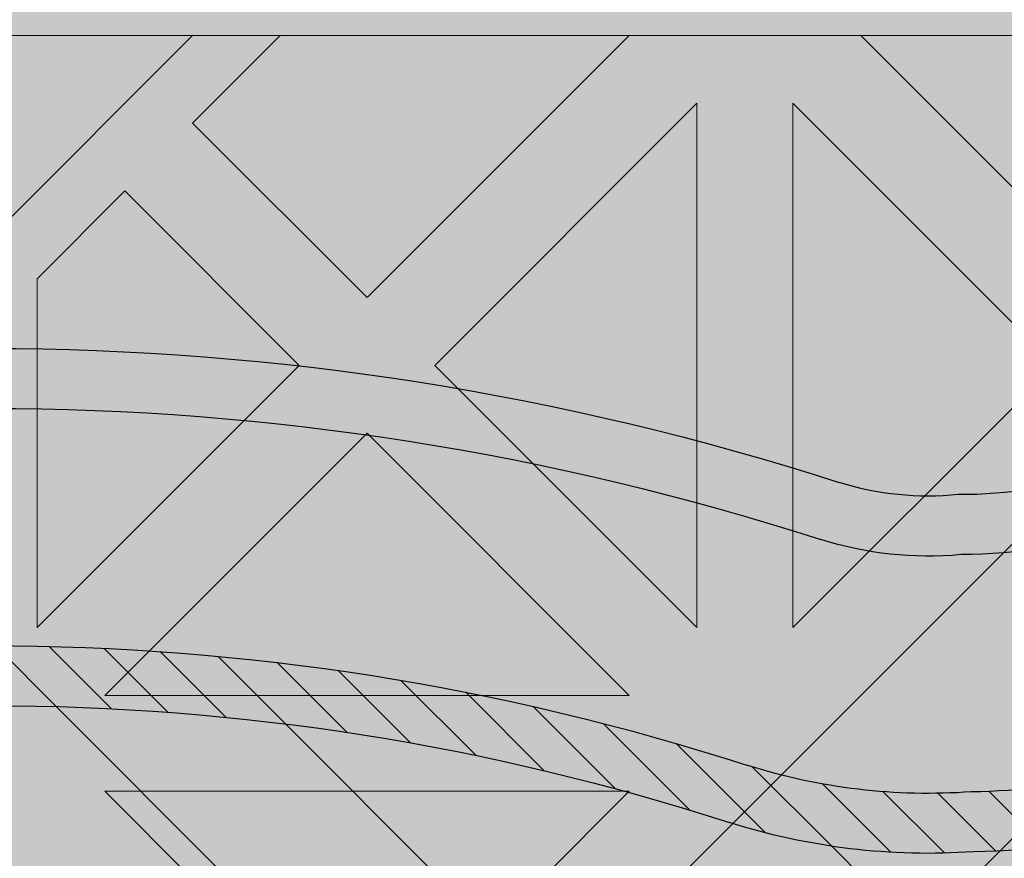
# Model space of a CAD drawing. Units: inches. Extents: x 844 to 2234, y 346 to 1084.
# Tile 81 of 93: x 2003.94 to 2006.557, y 708.742 to 710.971. Entities that reach past the tile are written whole.
import ezdxf

# ---------------------------------------------------------------- set-up
doc = ezdxf.new("R2010")
doc.units = ezdxf.units.IN
doc.header["$MEASUREMENT"] = 0
for name, color, linetype, lineweight in [('A-ANNO-DIMS', 2, 'Continuous', 18), ('furniture', 8, 'Continuous', 18), ('RA-AP-01$0$INT', 35, 'Continuous', 5)]:
    doc.layers.add(name, color=color, linetype=linetype, lineweight=lineweight)
doc.layers.add('RA-AP-01$0$FURN', color=3, linetype='Continuous')
doc.layers.add('RA-AP-01$0$WOOD', color=64, linetype='Continuous')
doc.styles.get("Standard").update_dxf_attribs({"font": 'arial.ttf'})
doc.dimstyles.get("Standard").update_dxf_attribs({"dimtxt": 6, "dimasz": 3, "dimexe": 0.18, "dimexo": 0.0625, "dimgap": 0.09, "dimtad": 0, "dimtih": 1, "dimtoh": 1, "dimdec": 1, "dimzin": 0, "dimdsep": 46, "dimlunit": 3, "dimtxsty": 'Standard', "dimblk": 'ARCHTICK', "dimcen": 0.09, "dimadec": 0, "dimazin": 0, "dimtfac": 1, "dimtdec": 1, "dimtofl": 0, "dimtmove": 0, "dimatfit": 3, "dimfxl": 1, "dimtolj": 1, "dimtzin": 0, "dimarcsym": 0})

# ---------------------------------------------------------------- blocks, each defined once
blk = doc.blocks.new('A$C18D01794')
at = {"layer": 'RA-AP-01$0$INT'}
blk.add_hatch(color=256, dxfattribs=at).paths.add_polyline_path([(4.505206456958071, -7.906712009588039), (5.305206456958072, -7.906712009588039), (5.305206456958072, -7.106712009588038), (5.255206456951893, -7.106712009588036), (5.25520645694868, -7.856712009570104), (4.555206456959269, -7.856712009588616), (4.555206456956052, -7.106712009588038), (4.505206456958073, -7.106712009588038)])
h = blk.add_hatch(color=256, dxfattribs=at)
h.paths.add_polyline_path([(4.585917135068448, -7.856712009587804), (4.614201406330596, -7.856712009587056), (4.668846067270487, -7.802067348644738), (4.723490728212344, -7.856712009584164), (4.771774999457151, -7.856712009582887), (4.826419660396886, -7.80206734864072), (4.862780050090322, -7.838427738332541), (4.844495778842715, -7.856712009580965), (4.862780050090411, -7.856712009580482), (4.905206456960182, -7.814285602707865), (4.947632863832445, -7.856712009578238), (4.965917135079675, -7.856712009577755), (4.947632863831759, -7.838427738330656), (4.983993253523576, -7.802067348637219), (5.038637914464627, -7.856712009575829), (5.08692218571208, -7.856712009574554), (5.141566846649976, -7.802067348634224), (5.196211507589851, -7.856712009571666), (5.224495778822615, -7.856712009570916), (4.905206456953975, -7.537422687702283)])
h.paths.add_polyline_path([(4.895206456956031, -7.575706958950402), (4.895206456958921, -7.684996280828174), (4.840561796018589, -7.630351619890275)], flags=16)
h.paths.add_polyline_path([(4.915206456955638, -7.575706958949956), (4.969851117895509, -7.630351619887399), (4.915206456957609, -7.684996280827732)], flags=16)
h.paths.add_polyline_path([(4.826419660395175, -7.644493755514321), (4.881064321335613, -7.699138416452331), (4.771774999456703, -7.69913841645522)], flags=16)
h.paths.add_polyline_path([(4.983993253519558, -7.644493755510815), (5.038637914460456, -7.699138416449285), (4.929348592581548, -7.69913841645126)], flags=16)
h.paths.add_polyline_path([(4.881064321336025, -7.719138416452334), (4.826419660397532, -7.773783077393256), (4.771774999457062, -7.719138416455217)], flags=16)
h.paths.add_polyline_path([(4.929348592582019, -7.71913841645126), (5.038637914460982, -7.719138416449284), (4.983993253522945, -7.773783077389749)], flags=16)
h.paths.add_polyline_path([(4.895206456960191, -7.733280552075633), (4.895206456962115, -7.806001331460164), (4.876922185715016, -7.824285602708492), (4.840561796021581, -7.787925213016675)], flags=16)
h.paths.add_polyline_path([(4.915206456958487, -7.733280552075187), (4.969851117899527, -7.787925213013798), (4.933490728206909, -7.824285602708034), (4.9152064569598, -7.806001331461736)], flags=16)
h.paths.add_polyline_path([(4.757632863832376, -7.733280552079264), (4.812277524772842, -7.787925213017304), (4.757632863834348, -7.842569873958233)], flags=16)
h.paths.add_polyline_path([(4.737632863832376, -7.73328055207979), (4.737632863834348, -7.842569873958701), (4.682988202893906, -7.787925213020692)], flags=16)
h.paths.add_polyline_path([(5.05278005008503, -7.733280552072701), (5.052780050087917, -7.842569873951664), (4.998135389146995, -7.787925213013169)], flags=16)
h.paths.add_polyline_path([(5.072780050085024, -7.733280552072333), (5.127424711025931, -7.787925213010806), (5.072780050087916, -7.842569873951244)], flags=16)
h.paths.add_polyline_path([(4.935917135072783, -7.506712009583784), (5.255206456948811, -7.826001331459767), (5.255206456948932, -7.797717060211899), (5.200561796010279, -7.743072399273238), (5.255206456949403, -7.688427738334128), (5.25520645694961, -7.640143467086677), (5.200561796009787, -7.585498806146837), (5.236922185702417, -7.549138416454212), (5.255206456949919, -7.56742268770172), (5.255206456949998, -7.549138416454178), (5.212780050078687, -7.506712009583814), (5.25520645695036, -7.464285602712145), (5.255206456950438, -7.446001331464763), (5.236922185702424, -7.464285602712779), (5.200561796009796, -7.427925213020149), (5.255206456950753, -7.373280552079203), (5.25520645695096, -7.324996280834394), (5.200561796010322, -7.270351619893748), (5.255206456951428, -7.215706958952649), (5.255206456951547, -7.187422687705071)])
h.paths.add_polyline_path([(5.042988202883395, -7.42792521302065), (5.097632863823085, -7.373280552080975), (5.097632863822622, -7.482569873959883)], flags=16)
h.paths.add_polyline_path([(5.028846067259663, -7.442067348644384), (5.083490728198774, -7.496712009583504), (4.974201406321001, -7.496712009583035)], flags=16)
h.paths.add_polyline_path([(5.117632863823087, -7.37328055208089), (5.172277524762331, -7.42792521302015), (5.11763286382262, -7.482569873959851)], flags=16)
h.paths.add_polyline_path([(5.08349072819877, -7.516712009582191), (5.028846067259652, -7.571356670521302), (4.974201406320998, -7.516712009582638)], flags=16)
h.paths.add_polyline_path([(5.131774999446817, -7.35913841645716), (5.186419660386065, -7.413783077396415), (5.241064321325782, -7.359138416456712)], flags=17)
h.paths.add_polyline_path([(5.131774999446228, -7.496712009583703), (5.186419660386065, -7.442067348643883), (5.222780050079488, -7.478427738337313), (5.204495778832781, -7.496712009584014)], flags=16)
h.paths.add_polyline_path([(5.097632863822613, -7.530854145205813), (5.097632863823061, -7.640143467084723), (5.042988202883383, -7.585498806145032)], flags=16)
h.paths.add_polyline_path([(5.131774999446899, -7.339138416457162), (5.241064321325809, -7.339138416456712), (5.186419660386591, -7.284493755517479)], flags=17)
h.paths.add_polyline_path([(5.131774999446226, -7.516712009581999), (5.204495778830767, -7.516712009581702), (5.22278005007868, -7.534996280829206), (5.186419660386049, -7.571356670521828)], flags=16)
h.paths.add_polyline_path([(5.11763286382262, -7.530854145205852), (5.17227752476232, -7.585498806145562), (5.117632863823064, -7.64014346708481)], flags=16)
h.paths.add_polyline_path([(5.186419660386069, -7.599640941770585), (5.241064321325754, -7.654285602710281), (5.131774999446791, -7.654285602709814)], flags=16)
h.paths.add_polyline_path([(5.131774999446872, -7.674285602709813), (5.24106432132578, -7.674285602710282), (5.186419660386554, -7.728930263649504)], flags=16)
h.paths.add_polyline_path([(5.255206456951811, -7.126001331467467), (5.255206456951895, -7.106712009588038), (4.555206456956052, -7.106712009588038), (4.555206456956136, -7.12600133146746), (4.905206456953973, -7.476001331465289)])
h.paths.add_polyline_path([(4.983993253513404, -7.368930263651977), (4.92934859257295, -7.314285602713969), (5.03863791445186, -7.314285602711063)], flags=16)
h.paths.add_polyline_path([(4.969851117889988, -7.383072399276016), (4.915206456952556, -7.437717060215906), (4.915206456949648, -7.328427738338133)], flags=16)
h.paths.add_polyline_path([(4.929348592572535, -7.294285602713971), (4.983993253511019, -7.239640941773039), (5.038637914451496, -7.294285602711065)], flags=16)
h.paths.add_polyline_path([(5.052780050074912, -7.280143467087016), (4.998135389134438, -7.225498806148989), (5.052780050072919, -7.170854145208052)], flags=16)
h.paths.add_polyline_path([(5.07278005007491, -7.280143467086489), (5.072780050072918, -7.170854145207579), (5.127424711013374, -7.225498806145578)], flags=16)
h.paths.add_polyline_path([(4.89520645695295, -7.437717060216355), (4.840561796013067, -7.383072399278919), (4.895206456950961, -7.328427738338582)], flags=16)
h.paths.add_polyline_path([(4.915206456948365, -7.280143467090674), (4.915206456946434, -7.207422687704125), (4.933490728192729, -7.18913841645701), (4.969851117886972, -7.225498806149623)], flags=16)
h.paths.add_polyline_path([(4.881064321327021, -7.314285602715054), (4.82641966038902, -7.368930263655506), (4.771774999448108, -7.314285602717047)], flags=16)
h.paths.add_polyline_path([(4.895206456950073, -7.280143467091125), (4.840561796009022, -7.225498806152518), (4.876922185700835, -7.18913841645908), (4.895206456948749, -7.207422687706589)], flags=16)
h.paths.add_polyline_path([(4.983993253510392, -7.211356670525576), (4.947632863816944, -7.174996280833758), (4.965917135064043, -7.156712009585847), (5.038637914448995, -7.156712009584522)], flags=16)
h.paths.add_polyline_path([(4.881064321326543, -7.294285602715056), (4.771774999447578, -7.294285602717046), (4.826419660385607, -7.239640941776569)], flags=16)
h.paths.add_polyline_path([(4.905206456946447, -7.19913841645844), (4.862780050074785, -7.156712009587725), (4.947632863816685, -7.156712009586302)], flags=16)
h.paths.add_polyline_path([(5.14156684663679, -7.211356670521528), (5.086922185696452, -7.156712009583639), (5.196211507574223, -7.156712009581651)], flags=16)
h.paths.add_polyline_path([(4.8264196603837, -7.211356670529104), (4.771774999442643, -7.156712009590501), (4.8444957788276, -7.156712009588568), (4.862780050075511, -7.17499628083566)], flags=16)
h.paths.add_polyline_path([(4.812277524760289, -7.225498806153156), (4.757632863822258, -7.28014346709363), (4.757632863819352, -7.170854145214669)], flags=16)
h.paths.add_polyline_path([(4.73763286382226, -7.280143467093997), (4.682988202881349, -7.22549880615554), (4.737632863819352, -7.170854145215086)], flags=16)
h.paths.add_polyline_path([(4.723490728195188, -7.156712009591787), (4.668846067257299, -7.211356670532127), (4.614201406317417, -7.156712009594693)], flags=16)
h.paths.add_polyline_path([(4.597632863829262, -7.506712009583814), (4.555206456957951, -7.54913841645418), (4.555206456958029, -7.56742268770172), (4.573490728205535, -7.549138416454212), (4.609851117898167, -7.585498806146839), (4.555206456958338, -7.640143467086675), (4.555206456958546, -7.688427738334125), (4.60985111789767, -7.743072399273238), (4.555206456959015, -7.797717060211899), (4.555206456959138, -7.826001331459767), (4.874495778835167, -7.506712009583786), (4.5552064569564, -7.187422687705062), (4.555206456956523, -7.215706958952644), (4.609851117897629, -7.270351619893746), (4.555206456956988, -7.324996280834396), (4.555206456957198, -7.373280552079195), (4.609851117898153, -7.427925213020147), (4.573490728205528, -7.464285602712779), (4.555206456957507, -7.446001331464756), (4.555206456957585, -7.464285602712143)])
h.paths.add_polyline_path([(4.712780050085332, -7.482569873959882), (4.712780050084863, -7.373280552080972), (4.767424711024555, -7.42792521302065)], flags=16)
h.paths.add_polyline_path([(4.726922185709173, -7.496712009583504), (4.781566846648288, -7.442067348644384), (4.836211507586949, -7.496712009583033)], flags=16)
h.paths.add_polyline_path([(4.692780050085327, -7.482569873959851), (4.638135389145619, -7.427925213020149), (4.692780050084865, -7.373280552080892)], flags=16)
h.paths.add_polyline_path([(4.726922185709182, -7.516712009582191), (4.836211507586949, -7.51671200958264), (4.7815668466483, -7.571356670521304)], flags=16)
h.paths.add_polyline_path([(4.678637914461726, -7.496712009583706), (4.605917135075169, -7.496712009584014), (4.587632863828464, -7.478427738337311), (4.623993253521887, -7.442067348643881)], flags=16)
h.paths.add_polyline_path([(4.712780050085336, -7.530854145205816), (4.767424711024568, -7.585498806145034), (4.71278005008489, -7.640143467084724)], flags=16)
h.paths.add_polyline_path([(4.678637914461726, -7.516712009582001), (4.623993253521899, -7.571356670521829), (4.587632863829271, -7.534996280829206), (4.605917135077185, -7.5167120095817)], flags=16)
h.paths.add_polyline_path([(4.692780050085336, -7.530854145205848), (4.692780050084889, -7.64014346708481), (4.638135389145632, -7.585498806145562)], flags=16)
h.paths.add_polyline_path([(4.623993253521885, -7.413783077396415), (4.678637914461131, -7.359138416457161), (4.56934859258217, -7.359138416456712)], flags=17)
h.paths.add_polyline_path([(4.623993253521901, -7.599640941770568), (4.678637914461158, -7.654285602709814), (4.569348592582195, -7.654285602710281)], flags=16)
h.paths.add_polyline_path([(4.678637914461051, -7.339138416457162), (4.623993253521361, -7.284493755517479), (4.569348592582143, -7.339138416456712)], flags=17)
h.paths.add_polyline_path([(4.678637914461076, -7.674285602709813), (4.623993253521399, -7.728930263649504), (4.569348592582167, -7.674285602710281)], flags=16)
h = blk.add_hatch(color=256, dxfattribs=at)
h.paths.add_polyline_path([(4.905206456954232, -7.537422687702028), (4.874495778835232, -7.506712009583718), (4.555206456959138, -7.826001331459766), (4.555206456959269, -7.856712009588616), (4.585917135068449, -7.856712009587804)])
h.paths.add_polyline_path([(4.935917135072152, -7.506712009583152), (4.905206456953497, -7.537422687701806), (5.224495778822614, -7.856712009570917), (5.255206456948681, -7.856712009570104), (5.255206456948813, -7.826001331459768)])
h.paths.add_polyline_path([(5.255206456951549, -7.18742268770507), (5.255206456951813, -7.126001331467461), (4.905206456953563, -7.476001331465701), (4.935917135072559, -7.506712009584006)])
h.paths.add_polyline_path([(4.874495778835167, -7.506712009583785), (4.905206456953818, -7.476001331465132), (4.555206456956135, -7.126001331467458), (4.555206456956399, -7.187422687705064)])
h = blk.add_hatch(color=256, dxfattribs=at)
h.paths.add_polyline_path([(4.969851117891331, -7.630351619889621), (4.915206456952669, -7.575706958950966), (4.915206456952222, -7.684996280828739)])
h.paths.add_polyline_path([(4.895206456953064, -7.575706958950968), (4.840561796014413, -7.630351619889628), (4.895206456953533, -7.684996280828741)])
h.paths.add_polyline_path([(4.826419660390684, -7.644493755513362), (4.771774999451003, -7.699138416453052), (4.881064321329913, -7.699138416452587)])
h.paths.add_polyline_path([(4.881064321329884, -7.719138416452585), (4.771774999450921, -7.719138416453052), (4.82641966039018, -7.773783077392298)])
h.paths.add_polyline_path([(4.895206456953734, -7.733280552076196), (4.840561796013912, -7.787925213016031), (4.876922185707337, -7.824285602709455), (4.895206456954043, -7.806001331462747)])
h.paths.add_polyline_path([(4.862780050082808, -7.838427738332388), (4.826419660390178, -7.802067348639763), (4.771774999450351, -7.856712009579595), (4.844495778835303, -7.856712009579895)])
h.paths.add_polyline_path([(4.812277524766446, -7.787925213016036), (4.757632863827191, -7.733280552076788), (4.757632863826741, -7.842569873955747)])
h.paths.add_polyline_path([(4.737632863827191, -7.733280552076863), (4.682988202887508, -7.787925213016558), (4.737632863826743, -7.842569873955778)])
h.paths.add_polyline_path([(4.668846067263777, -7.802067348640287), (4.614201406325123, -7.856712009578949), (4.723490728202894, -7.856712009579402)])
h.paths.add_polyline_path([(4.905206456953846, -7.814285602708654), (4.862780050082654, -7.856712009579847), (4.947632863824561, -7.85671200958032)])
h.paths.add_polyline_path([(4.915206456952028, -7.733280552076195), (4.91520645695173, -7.806001331460731), (4.933490728199234, -7.824285602708648), (4.96985111789186, -7.787925213016022)])
h.paths.add_polyline_path([(5.038637914454841, -7.719138416453029), (4.929348592575874, -7.71913841645258), (4.983993253515593, -7.773783077392289)])
h.paths.add_polyline_path([(4.983993253515065, -7.644493755513352), (4.929348592575849, -7.699138416452582), (5.038637914454755, -7.699138416453031)])
h.paths.add_polyline_path([(5.052780050079843, -7.73328055207676), (4.998135389140595, -7.787925213016018), (5.052780050080309, -7.842569873955721)])
h.paths.add_polyline_path([(4.983993253516868, -7.802067348639752), (4.947632863824241, -7.838427738332383), (4.965917135071747, -7.856712009579888), (5.038637914456701, -7.856712009579572)])
h.paths.add_polyline_path([(5.127424711019533, -7.787925213016519), (5.072780050079843, -7.733280552076838), (5.07278005008031, -7.842569873955751)])
h.paths.add_polyline_path([(5.141566846643269, -7.802067348640248), (5.086922185704154, -7.85671200957937), (5.196211507581929, -7.856712009578901)])
for p, q in [((4.874495778835167, -7.506712009583786), (4.555206456959136, -7.826001331459769)), ((4.905206456953975, -7.537422687702283), (4.585917135071132, -7.856712009585121)), ((4.826419660395171, -7.644493755514321), (4.771774999456703, -7.69913841645522)), ((4.881064321335613, -7.699138416452333), (4.826419660395173, -7.64449375551432)), ((4.771774999456703, -7.69913841645522), (4.881064321335613, -7.699138416452333)), ((4.771774999457064, -7.719138416455219), (4.881064321336027, -7.719138416452333)), ((4.771774999457064, -7.719138416455219), (4.826419660397532, -7.773783077393256)), ((4.881064321336027, -7.719138416452333), (4.826419660397532, -7.773783077393256)), ((4.682988202893908, -7.78792521302069), (4.737632863832376, -7.733280552079792)), ((4.737632863832376, -7.733280552079792), (4.737632863834348, -7.842569873958701)), ((4.757632863832376, -7.733280552079266), (4.812277524772842, -7.787925213017302)), ((4.757632863832376, -7.733280552079266), (4.757632863834348, -7.842569873958229)), ((4.895206456960191, -7.73328055207563), (4.840561796021581, -7.787925213016675)), ((4.895206456962113, -7.806001331460581), (4.895206456960191, -7.73328055207563)), ((4.737632863834348, -7.842569873958701), (4.682988202893906, -7.787925213020692)), ((4.757632863834348, -7.842569873958229), (4.812277524772842, -7.787925213017302)), ((4.840561796021581, -7.787925213016674), (4.876922185715016, -7.824285602708492)), ((4.723490728210815, -7.856712009582635), (4.668846067270487, -7.802067348644737)), ((4.771774999458274, -7.856712009581762), (4.826419660396887, -7.80206734864072)), ((4.826419660396886, -7.80206734864072), (4.862780050090322, -7.838427738332541)), ((4.895206456959797, -7.806001331462484), (4.876922185715016, -7.824285602708492)), ((4.905206456960184, -7.814285602707865), (4.862780050090411, -7.856712009580478)), ((4.844495778843225, -7.856712009580453), (4.862780050090324, -7.838427738332541)), ((4.555206456959269, -7.856712009588616), (5.255206456948681, -7.856712009570104)), ((4.844495778843225, -7.856712009580451), (4.771774999458274, -7.856712009581762)), ((4.947632863832319, -7.856712009578112), (4.862780050090411, -7.856712009580478))]:
    blk.add_line(p, q, dxfattribs=at)
blk = doc.blocks.new('A$C32926AE1')
at = {"layer": 'RA-AP-01$0$WOOD'}
h = blk.add_hatch(color=256, dxfattribs=at)
h.dxf.hatch_style = 1
h.paths.add_polyline_path([(5.157430609644524, 4.573483066760929, -0.1009492694046607), (5.155401577623758, 4.593365984175333, -0.1842662638101597), (5.172249623284174, 4.638795604568598, 0.2056608120311276), (5.179560981299304, 4.661316324430096, 0.3614336704623542), (5.134352340494423, 4.706524965234944, 0.2056608120311297), (5.111831620632933, 4.699213607219793, -0.1842662638101113), (5.066402000239693, 4.682365561559342, -0.1055311479399994), (5.045656153913092, 4.68467289944697, 0.1567636581983829), (4.763886414745334, 4.684672899446966, -0.1055311479399895), (4.743140568418733, 4.68236556155934, -0.1842662638100833), (4.6977109480255, 4.69921360721979, 0.2056608120302612), (4.675190228164109, 4.706524965234949, 0.3614336704708441), (4.629981587358889, 4.66131632442871, 0.2056608120245944), (4.637292945374126, 4.638795604567974, -0.1842662638101024), (4.654140991034615, 4.59336598417475, -0.1009492694055169), (4.652111959013835, 4.573483066760181, 0.021410119221476), (4.629748025606143, 4.156712009541676, 0.0214101192214795), (4.652111959013809, 3.739940952323101, -0.1009492694059586), (4.654140991034615, 3.720058034908448, -0.1842662638100975), (4.637292945374126, 3.674628414515226, 0.2056608120245705), (4.629981587358889, 3.652107694654492, 0.3614336704708879), (4.675190228164113, 3.606899053848249, 0.2056608120302384), (4.697710948025501, 3.614210411863408, -0.1842662638100995), (4.743140568418738, 3.63105845752386, -0.1055311479402541), (4.763886414745388, 3.628751119636215, 0.1567636581983776), (5.045656153913137, 3.628751119636244, -0.1055311479397538), (5.066402000239692, 3.631058457523857, -0.1842662638101067), (5.111831620632931, 3.614210411863407, 0.2056608120310924), (5.134352340494417, 3.606899053848256, 0.3614336704624001), (5.179560981299307, 3.652107694653103, 0.2056608120311314), (5.172249623284175, 3.6746284145146, -0.1842662638101402), (5.155401577623758, 3.72005803490786, -0.1009492694051366), (5.15743060964455, 3.739940952322354, 0.0214101192215073), (5.179794543052287, 4.156712009541468, 0.0214101192215252)])
h.paths.add_polyline_path([(4.639748609479751, 4.156712009541513, 0.0213537860821624), (4.661970494867118, 3.741887061152232, -0.094075836301374), (4.664143710413708, 3.7196126951003, -0.1824818158568985), (4.644813765429836, 3.668037719127816, 0.2056608120245319), (4.639939526753007, 3.653023905887301, 0.3614336704710246), (4.676106439397173, 3.616856993242342, 0.2056608120302234), (4.691120252638095, 3.621731231919122, -0.1824818158602558), (4.742695228611606, 3.641061176902986, -0.1029891339458722), (4.766991894714349, 3.638256818950944, 0.156709409989566), (5.042550673941472, 3.638256818950105, -0.102989133958497), (5.066847340047078, 3.641061176902949, -0.1824818158594995), (5.118422316020358, 3.621731231919103, 0.2056608120311416), (5.133436129261316, 3.616856993242346, 0.3614336704621468), (5.169603041905217, 3.653023905886178, 0.2056608120310986), (5.164728803228477, 3.668037719127177, -0.1824818158565612), (5.145398858244737, 3.719612695099578, -0.0940758363009313), (5.147572073791232, 3.741887061151398, 0.0213537860822023), (5.169793959178681, 4.156712009541451, 0.0213537860822226), (5.147572073791203, 4.571536957931898, -0.0940758363005034), (5.145398858244737, 4.59381132398362, -0.1824818158565587), (5.164728803228476, 4.645386299956021, 0.2056608120311045), (5.169603041905216, 4.66040011319702, 0.3614336704621845), (5.133436129261313, 4.696567025840856, 0.2056608120310773), (5.118422316020359, 4.691692787164098, -0.182481815859508), (5.066847340047078, 4.67236284218025, -0.1029891339584606), (5.04255067394148, 4.675167200133092, 0.156709409989566), (4.766991894714357, 4.675167200132257, -0.1029891339458842), (4.742695228611611, 4.672362842180213, -0.1824818158602725), (4.691120252638095, 4.691692787164077, 0.2056608120302152), (4.676106439397174, 4.696567025840858, 0.3614336704710363), (4.639939526753005, 4.660400113195899, 0.2056608120245495), (4.644813765429837, 4.645386299955384, -0.1824818158568934), (4.664143710413708, 4.593811323982902, -0.0940758363009187), (4.661970494867149, 4.571536957931074, 0.021353786082177)], flags=16)
h.paths.add_polyline_path([(5.129794543052235, 4.432167055276933, -0.0141661062790638), (5.130152669293814, 4.156927903047693, -0.0141661062790647), (5.129794543052234, 3.881688750818433, -0.0785247771143638), (5.10979738006795, 3.755143611847103, 0.0945969212073497), (5.105408519571111, 3.717898134952927, 0.1043170707844957), (5.116074640131521, 3.670385395016088, 0.1043170707864965), (5.068561900193738, 3.681051515576561, 0.09459692119553), (5.031316423304057, 3.676662655080835, -0.1580239521427272), (4.778226145355827, 3.676662655080367, 0.0945969211986668), (4.740980668464973, 3.681051515576592, 0.1043170707882822), (4.693467928526415, 3.670385395015844, 0.1043170707867916), (4.704134049087309, 3.717898134953662, 0.0945969211972894), (4.69974518859162, 3.755143611844042, -0.0785247771163196), (4.679748025606343, 3.881688750818406, -0.0141661062790663), (4.679389899364763, 4.156927903047693, -0.0141661062790672), (4.679748025606343, 4.432167055276998, -0.0785247771163064), (4.699745188591625, 4.55871219425134, 0.094596921197333), (4.704134049087308, 4.595957671141738, 0.1043170707867205), (4.693467928526416, 4.643470411079523, 0.1043170707882628), (4.740980668464965, 4.632804290518776, 0.0945969211988114), (4.778226145355874, 4.637193151015016, -0.158023952142669), (5.031316423304015, 4.637193151014546, 0.0945969211956361), (5.068561900193736, 4.632804290518806, 0.1043170707864979), (5.11607464013152, 4.643470411079278, 0.1043170707844617), (5.105408519571112, 4.595957671142455, 0.0945969212074597), (5.109797380067959, 4.558712194248236, -0.0785247771143467)], flags=0)
h.paths.add_polyline_path([(5.119794532311105, 4.432259799204851, -0.0142000800617244), (5.120156169157484, 4.156927903047701, -0.0142000800617277), (5.119794532311105, 3.881596006890482, -0.0784894509520253), (5.100273383573699, 3.758192358677797, 0.0940138827242913), (5.095413455884425, 3.717477693979438, 0.0606271852308753), (5.099615656341024, 3.686844378806616, 0.0606271852322524), (5.068982341167493, 3.691046579263239, 0.0940138827010453), (5.028267676478798, 3.686186651576848, -0.1580706864508061), (4.781274892180912, 3.686186651576435, 0.0940138827026903), (4.740560227491556, 3.691046579263279, 0.0606271852339895), (4.709926912317155, 3.686844378806508, 0.0606271852329405), (4.714129112773991, 3.717477693980356, 0.094013882701304), (4.709269185087677, 3.758192358669163, -0.0784894509577193), (4.689748036347473, 3.881596006890469, -0.014200080061729), (4.689386399501094, 4.156927903047709, -0.0142000800617217), (4.689748036347473, 4.432259799204808, -0.078489450957724), (4.709269185087651, 4.555663447426125, 0.0940138827014585), (4.714129112773992, 4.596378112114996, 0.0606271852329731), (4.709926912317154, 4.62701142728886, 0.0606271852340196), (4.74056022749157, 4.622809226832087, 0.0940138827024997), (4.781274892180847, 4.627669154518912, -0.1580706864508359), (5.028267676478777, 4.627669154518526, 0.0940138827010946), (5.068982341167492, 4.622809226832129, 0.060627185232254), (5.099615656341024, 4.627011427288751, 0.0606271852308727), (5.095413455884425, 4.59637811211593, 0.0940138827241088), (5.100273383573675, 4.555663447417647, -0.0784894509520978)], flags=0)
h.paths.add_polyline_path([(5.06978912287499, 4.430218106756144, -0.014241683694547), (5.070173729147532, 4.156927903047672, -0.0142416836945458), (5.06978912287499, 3.883637699339223, -0.0800609523125196), (5.052662118612511, 3.773463122773442, 0.0526421978001116), (5.04590916754064, 3.740550867606997, 0.0526421977992423), (5.012996912374707, 3.73379791653534, -0.1583028414718258), (4.796545656286308, 3.73379791653451, 0.0526421978034211), (4.763633401117837, 3.740550867607021, 0.0526421978018622), (4.756880450045755, 3.773463122774558, -0.0800609523117106), (4.739753445783639, 3.883637699339268, -0.0142416836945435), (4.739368839511098, 4.156927903047671, -0.0142416836945477), (4.739753445783639, 4.430218106756155, -0.0800609523116345), (4.75688045004574, 4.540392683320762, 0.052642197801941), (4.763633401117837, 4.573304938488346, 0.0526421978035071), (4.796545656286361, 4.580057889560873, -0.1583028414717561), (5.012996912374669, 4.580057889560039, 0.0526421977993048), (5.04590916754064, 4.57330493848837, 0.0526421978002057), (5.052662118612529, 4.540392683321868, -0.080060952312477)], flags=0)
h.paths.add_polyline_path([(5.049789715110557, 4.43038092723357, -0.0143097550741839), (5.05018085590259, 4.156927903047715, -0.0143097550741854), (5.049789715110558, 3.883474878861827, -0.0800685599149176), (5.03362098255317, 3.779581877367999, 0.0306258898956367), (5.028241146483733, 3.758218888663947, 0.0306258898977031), (5.006878157778253, 3.75283905259408, -0.1583983521624096), (4.802664410878162, 3.752839052594731, 0.0306258898946014), (4.781301422174808, 3.758218888663924, 0.0306258898967912), (4.775921586105202, 3.779581877368794, -0.080068559914251), (4.759752853548071, 3.883474878861786, -0.0143097550741854), (4.759361712756037, 4.156927903047671, -0.0143097550741854), (4.759752853548071, 4.430380927233557, -0.0800685599142479), (4.775921586105193, 4.534273928726546, 0.0306258898968306), (4.781301422174808, 4.555636917431444, 0.0306258898945754), (4.802664410878143, 4.561016753500631, -0.1583983521624168), (5.006878157778244, 4.561016753501291, 0.0306258898977177), (5.028241146483733, 4.555636917431421, 0.0306258898958182), (5.03362098255321, 4.534273928727244, -0.080068559914796)], flags=0)
h.paths.add_polyline_path([(4.999766070382627, 4.428171244713864, -0.0143443147609634), (5.000198441819402, 4.156927903047689, -0.0143443147609612), (4.999766070382627, 3.885684561381556, -0.0784641635803329), (4.987356730658798, 3.799103304488872, -0.1506053783831347), (4.822185837999821, 3.79910330448882, -0.0784641635803318), (4.809776498276007, 3.885684561381509, -0.014344314760963), (4.809344126839227, 4.156927903047677, -0.0143443147609645), (4.809776498276007, 4.428171244713873, -0.0784641635803192), (4.822185837999822, 4.514752501606549, -0.1506053783831338), (4.987356730658798, 4.514752501606494, -0.078464163580285)], flags=0)
h.paths.add_polyline_path([(4.979755254238824, 4.42764379880488, -0.0143772539198268), (4.980205517789977, 4.156927903047693, -0.0143772539198275), (4.979755254238824, 3.886212007290489, -0.0689242507424422), (4.971183264704897, 3.815276770442801, -0.1296645318904179), (4.838359303953726, 3.815276770442746, -0.0689242507424186), (4.829787314419809, 3.886212007290419, -0.0143772539198292), (4.829337050868653, 4.156927903047653, -0.0143772539198325), (4.829787314419809, 4.427643798804946, -0.0689242507424211), (4.838359303953725, 4.498579035652621, -0.1296645318904187), (4.971183264704897, 4.498579035652565, -0.0689242507424401)], flags=0)
h = blk.add_hatch(color=256, dxfattribs=at)
h.dxf.hatch_style = 1
h.paths.add_polyline_path([(5.145398858244737, 4.59381132398362, -0.1824818158565616), (5.164728803228476, 4.645386299956021, 0.2056608120311045), (5.169603041905216, 4.66040011319702, 0.3614336704621845), (5.133436129261313, 4.696567025840856, 0.2056608120310773), (5.118422316020359, 4.691692787164098, -0.182481815859508), (5.066847340047078, 4.67236284218025, -0.1029891339584606), (5.04255067394148, 4.675167200133092, 0.156709409989566), (4.766991894714357, 4.675167200132257, -0.1029891339458842), (4.742695228611611, 4.672362842180213, -0.1824818158602725), (4.691120252638095, 4.691692787164077, 0.2056608120302152), (4.676106439397174, 4.696567025840858, 0.3614336704710363), (4.639939526753005, 4.660400113195899, 0.2056608120245495), (4.644813765429837, 4.645386299955384, -0.1824818158568934), (4.664143710413708, 4.593811323982902, -0.0940758363009187), (4.661970494867149, 4.571536957931074, 0.0213537860821772), (4.639748609479751, 4.156712009541507, 0.0213537860821625), (4.661970494867119, 3.741887061152226, -0.0940758363013071), (4.664143710413708, 3.719612695100309, -0.1824818158569294), (4.644813765429836, 3.668037719127816, 0.2056608120245319), (4.639939526753007, 3.653023905887301, 0.3614336704710246), (4.676106439397173, 3.616856993242342, 0.2056608120302234), (4.691120252638095, 3.621731231919122, -0.1824818158602558), (4.742695228611606, 3.641061176902986, -0.1029891339458722), (4.766991894714349, 3.638256818950944, 0.156709409989566), (5.042550673941472, 3.638256818950105, -0.102989133958497), (5.066847340047078, 3.641061176902949, -0.1824818158594995), (5.118422316020358, 3.621731231919103, 0.2056608120311416), (5.133436129261316, 3.616856993242346, 0.3614336704621468), (5.169603041905217, 3.653023905886178, 0.2056608120310986), (5.164728803228477, 3.668037719127177, -0.1824818158565612), (5.145398858244737, 3.719612695099578, -0.0940758363009313), (5.147572073791232, 3.741887061151398, 0.0213537860822023), (5.169793959178681, 4.156712009541451, 0.0213537860822226), (5.147572073791203, 4.571536957931898, -0.0940758363004996)])
h.paths.add_polyline_path([(5.109797380067958, 4.55871219424824, -0.0785247771143472), (5.129794543052234, 4.432167055276936, -0.0141661062790644), (5.130152669293814, 4.156927903047685, -0.014166106279066), (5.129794543052234, 3.881688750818401, -0.0785247771143517), (5.109797380067946, 3.755143611847092, 0.0945969212073132), (5.105408519571111, 3.717898134952929, 0.1043170707844995), (5.116074640131521, 3.670385395016088, 0.1043170707864965), (5.068561900193738, 3.681051515576561, 0.09459692119553), (5.031316423304057, 3.676662655080835, -0.1580239521427272), (4.778226145355827, 3.676662655080367, 0.0945969211986668), (4.740980668464973, 3.681051515576592, 0.1043170707882822), (4.693467928526415, 3.670385395015844, 0.1043170707867916), (4.704134049087309, 3.717898134953662, 0.0945969211972894), (4.69974518859162, 3.755143611844042, -0.0785247771163196), (4.679748025606343, 3.881688750818406, -0.0141661062790663), (4.679389899364763, 4.156927903047693, -0.0141661062790672), (4.679748025606343, 4.432167055276998, -0.0785247771163064), (4.699745188591625, 4.55871219425134, 0.094596921197333), (4.704134049087308, 4.595957671141738, 0.1043170707867205), (4.693467928526416, 4.643470411079523, 0.1043170707882628), (4.740980668464965, 4.632804290518776, 0.0945969211988114), (4.778226145355874, 4.637193151015016, -0.158023952142669), (5.031316423304015, 4.637193151014546, 0.0945969211956361), (5.068561900193736, 4.632804290518806, 0.1043170707864979), (5.11607464013152, 4.643470411079278, 0.1043170707844617), (5.105408519571112, 4.595957671142455, 0.0945969212074504)], flags=16)
h.paths.add_polyline_path([(5.100273383573655, 4.55566344741771, -0.0784894509521388), (5.119794532311105, 4.432259799204852, -0.0142000800617252), (5.120156169157484, 4.156927903047686, -0.014200080061726), (5.119794532311105, 3.881596006890502, -0.0784894509520446), (5.100273383573696, 3.758192358677786, 0.0940138827242721), (5.095413455884425, 3.717477693979436, 0.0606271852308692), (5.099615656341024, 3.686844378806616, 0.0606271852322522), (5.068982341167493, 3.691046579263239, 0.0940138827010453), (5.028267676478798, 3.686186651576848, -0.1580706864508061), (4.781274892180912, 3.686186651576435, 0.0940138827026903), (4.740560227491556, 3.691046579263279, 0.0606271852339895), (4.709926912317155, 3.686844378806508, 0.0606271852329405), (4.714129112773991, 3.717477693980356, 0.094013882701304), (4.709269185087677, 3.758192358669163, -0.0784894509577193), (4.689748036347473, 3.881596006890469, -0.014200080061729), (4.689386399501094, 4.156927903047709, -0.0142000800617217), (4.689748036347473, 4.432259799204808, -0.078489450957724), (4.709269185087651, 4.555663447426125, 0.0940138827014585), (4.714129112773992, 4.596378112114996, 0.0606271852329731), (4.709926912317154, 4.62701142728886, 0.0606271852340196), (4.74056022749157, 4.622809226832087, 0.0940138827024997), (4.781274892180847, 4.627669154518912, -0.1580706864508359), (5.028267676478777, 4.627669154518526, 0.0940138827010946), (5.068982341167492, 4.622809226832129, 0.060627185232254), (5.099615656341024, 4.627011427288751, 0.0606271852308727), (5.095413455884425, 4.59637811211593, 0.094013882723957)], flags=0)
h.paths.add_polyline_path([(5.04590916754064, 4.57330493848837, 0.0526421978002057), (5.052662118612529, 4.540392683321868, -0.0800609523124783), (5.06978912287499, 4.430218106756142, -0.0142416836945469), (5.070173729147532, 4.156927903047672, -0.0142416836945458), (5.06978912287499, 3.883637699339223, -0.0800609523125196), (5.052662118612511, 3.773463122773442, 0.0526421978001116), (5.04590916754064, 3.740550867606997, 0.0526421977992423), (5.012996912374707, 3.73379791653534, -0.1583028414718258), (4.796545656286308, 3.73379791653451, 0.0526421978034211), (4.763633401117837, 3.740550867607021, 0.0526421978018622), (4.756880450045755, 3.773463122774558, -0.0800609523117106), (4.739753445783639, 3.883637699339268, -0.0142416836945435), (4.739368839511098, 4.156927903047671, -0.0142416836945477), (4.739753445783639, 4.430218106756155, -0.0800609523116345), (4.75688045004574, 4.540392683320762, 0.052642197801941), (4.763633401117837, 4.573304938488346, 0.0526421978035071), (4.796545656286361, 4.580057889560873, -0.1583028414717561), (5.012996912374669, 4.580057889560039, 0.0526421977993048)], flags=0)
h.paths.add_polyline_path([(5.028241146483733, 4.555636917431422, 0.0306258898956949), (5.033620982553182, 4.534273928727329, -0.0800685599148649), (5.049789715110557, 4.430380927233569, -0.0143097550741839), (5.05018085590259, 4.156927903047715, -0.0143097550741854), (5.049789715110558, 3.883474878861827, -0.0800685599149176), (5.03362098255317, 3.779581877367999, 0.0306258898956367), (5.028241146483733, 3.758218888663947, 0.0306258898977031), (5.006878157778253, 3.75283905259408, -0.1583983521624096), (4.802664410878162, 3.752839052594731, 0.0306258898946014), (4.781301422174808, 3.758218888663924, 0.0306258898967912), (4.775921586105202, 3.779581877368794, -0.080068559914251), (4.759752853548071, 3.883474878861786, -0.0143097550741854), (4.759361712756037, 4.156927903047671, -0.0143097550741854), (4.759752853548071, 4.430380927233557, -0.0800685599142479), (4.775921586105193, 4.534273928726546, 0.0306258898968306), (4.781301422174808, 4.555636917431444, 0.0306258898945754), (4.802664410878143, 4.561016753500631, -0.1583983521624168), (5.006878157778244, 4.561016753501291, 0.0306258898977174)], flags=0)
h.paths.add_polyline_path([(4.987356730658798, 4.514752501606494, -0.0784641635803018), (4.999766070382627, 4.428171244713845, -0.0143443147609637), (5.000198441819402, 4.156927903047665, -0.0143443147609622), (4.999766070382628, 3.885684561381514, -0.0784641635802952), (4.987356730658797, 3.799103304488872, -0.1506053783831338), (4.822185837999821, 3.799103304488819, -0.0784641635803342), (4.809776498276007, 3.885684561381512, -0.0143443147609628), (4.809344126839227, 4.156927903047676, -0.0143443147609646), (4.809776498276007, 4.428171244713873, -0.0784641635803192), (4.822185837999822, 4.514752501606549, -0.1506053783831338)], flags=0)
h.paths.add_polyline_path([(4.971183264704897, 4.498579035652566, -0.0689242507424384), (4.979755254238824, 4.427643798804883, -0.0143772539198276), (4.980205517789977, 4.15692790304768, -0.0143772539198258), (4.979755254238823, 3.88621200729051, -0.0689242507424628), (4.971183264704897, 3.815276770442801, -0.129664531890417), (4.838359303953726, 3.815276770442746, -0.0689242507424186), (4.829787314419809, 3.886212007290419, -0.0143772539198292), (4.829337050868653, 4.156927903047653, -0.0143772539198325), (4.829787314419809, 4.427643798804946, -0.0689242507424211), (4.838359303953725, 4.498579035652621, -0.1296645318904187)], flags=0)
h = blk.add_hatch(dxfattribs=at)
h.set_pattern_fill('ANSI31', color=256, scale=0.05, style=0)
h.set_pattern_definition([(45, (0, 0), (-0.0044194173824159, 0.0044194173824159), [])])
h.paths.add_polyline_path([(5.130152669293814, 4.156927903047704, 0.0141661062790657), (5.129794543052234, 4.432167055276982, 0.0777827904001433), (5.110168979996553, 4.557559993161921, -0.0976515123401879), (5.105408519571111, 4.595957671142454, -0.1043170707844687), (5.116074640131522, 4.64347041107928), (5.099615656341024, 4.627011427288751, 0.0606271852308727), (5.095413455884425, 4.59637811211593, 0.0940138827241088), (5.100273383573675, 4.555663447417647, -0.0784894509520972), (5.119794532311105, 4.432259799204852, -0.0142000800617252), (5.120156169157484, 4.156927903047686, -0.014200080061726), (5.119794532311105, 3.881596006890502, -0.0784894509520446), (5.100273383573696, 3.758192358677786, 0.0940138827242721), (5.095413455884425, 3.717477693979436, 0.0606271852308692), (5.099615656341024, 3.686844378806616), (5.116074640131519, 3.67038539501609, -0.1043170707844594), (5.105408519571112, 3.717898134952912, -0.0976515123401594), (5.11016897999655, 3.756295812933435, 0.0777827904001654), (5.129794543052234, 3.881688750818409, 0.0141661062790665)])
h.paths.add_polyline_path([(5.030164222210597, 3.676291055149937, -0.0976515123472002), (5.068561900193739, 3.681051515576561, -0.1043170707864927), (5.116074640131521, 3.670385395016088), (5.099615656341024, 3.686844378806616, 0.0606271852322522), (5.068982341167493, 3.691046579263239, 0.0940138827010453), (5.028267676478798, 3.686186651576848, -0.1580706864508061), (4.781274892180912, 3.686186651576435, 0.0940138827026903), (4.740560227491556, 3.691046579263279, 0.0606271852339913), (4.709926912317154, 3.686844378806508), (4.693467928526416, 3.670385395015845, -0.1043170707882796), (4.740980668464973, 3.681051515576592, -0.0976515123427246), (4.779378346446416, 3.676291055150394, 0.156512506893803)])
h.paths.add_polyline_path([(4.689748036347473, 3.881596006890472, -0.014200080061729), (4.689386399501094, 4.156927903047712, -0.0142000800617195), (4.689748036347473, 4.432259799204768, -0.078489450957742), (4.709269185087648, 4.555663447426114, 0.0940138827014821), (4.714129112773992, 4.596378112114995, 0.0606271852329748), (4.709926912317154, 4.62701142728886), (4.693467928526414, 4.643470411079524, -0.1043170707867939), (4.704134049087309, 4.595957671141706, -0.09765151234893), (4.699373588660725, 4.557559993157876, 0.0777827903975372), (4.679748025606343, 4.432167055276987, 0.0141661062790675), (4.679389899364763, 4.156927903047675, 0.0141661062790641), (4.679748025606343, 3.88168875081843, 0.0777827903975637), (4.699373588660724, 3.756295812937497, -0.0976515123490278), (4.704134049087308, 3.717898134953629, -0.1043170707867196), (4.693467928526416, 3.670385395015845), (4.709926912317155, 3.686844378806508, 0.0606271852329413), (4.714129112773991, 3.717477693980357, 0.0940138827013084), (4.709269185087676, 3.758192358669166, -0.0784894509577192)])
h.paths.add_polyline_path([(4.779378346446434, 4.63756475094498, -0.0976515123427943), (4.740980668464964, 4.632804290518776, -0.1043170707882609), (4.693467928526416, 4.643470411079523), (4.709926912317154, 4.62701142728886, 0.0606271852340196), (4.74056022749157, 4.622809226832087, 0.0940138827024997), (4.781274892180847, 4.627669154518912, -0.1580706864508359), (5.028267676478777, 4.627669154518526, 0.0940138827010946), (5.068982341167492, 4.622809226832129, 0.060627185232254), (5.099615656341024, 4.627011427288751), (5.116074640131521, 4.643470411079279, -0.1043170707865022), (5.068561900193735, 4.632804290518806, -0.0976515123475899), (5.030164222210446, 4.637564750945479, 0.1565125068936924)])
h = blk.add_hatch(dxfattribs=at)
h.set_pattern_fill('ANSI32', color=256, scale=0.2, style=0)
h.set_pattern_definition([(45, (0, 0), (-0.0530330085889911, 0.0530330085889911), []), (45, (0.035355339, 0), (-0.0530330085889911, 0.0530330085889911), [])])
h.paths.add_polyline_path([(5.119794532311105, 4.432259799204823, 0.0777015974868765), (5.10065834347252, 4.554469821747928, -0.0968902511992216), (5.095413455884425, 4.596378112115931, -0.060627185230871), (5.099615656341024, 4.627011427288751, -0.060627185232254), (5.068982341167492, 4.622809226832129, -0.0968902512198245), (5.027074050790956, 4.628054114423209, 0.1564657949319105), (4.782468517866163, 4.628054114422785, -0.0968902512152247), (4.740560227491555, 4.622809226832088, -0.0606271852339878), (4.709926912317155, 4.627011427288859, -0.0606271852329413), (4.714129112773991, 4.596378112115011, -0.0968902512205338), (4.708884225182929, 4.554469821738175, 0.0777015974804443), (4.689748036347473, 4.43225979920482, 0.0142000800617215), (4.689386399501094, 4.156927903047726, 0.0142000800617273), (4.689748036347473, 3.88159600689052, 0.077701597480541), (4.708884225182985, 3.759385984357019, -0.096890251220082), (4.714129112773992, 3.717477693980371, -0.0606271852329731), (4.709926912317154, 3.686844378806507, -0.060627185233988), (4.740560227491554, 3.691046579263279, -0.0968902512152569), (4.782468517866175, 3.685801691672578, 0.1564657949319236), (5.027074050790988, 3.685801691672169, -0.0968902512197451), (5.068982341167491, 3.691046579263239, -0.0606271852322557), (5.099615656341024, 3.686844378806616, -0.0606271852308727), (5.095413455884425, 3.717477693979438, -0.0968902511991229), (5.100658343472507, 3.7593859843474, 0.0777015974868745), (5.119794532311105, 3.8815960068905, 0.014200080061726), (5.120156169157484, 4.156927903047685, 0.0142000800617238)])
h.paths.add_polyline_path([(5.070173729147531, 4.156927903047684, -0.0142416836945481), (5.06978912287499, 3.883637699339191, -0.0800609523125107), (5.052662118612505, 3.773463122773424, 0.0526421978000811), (5.04590916754064, 3.740550867606997, 0.0526421977993214), (5.012996912374658, 3.733797916535325, -0.1583028414717916), (4.796545656286304, 3.733797916534512, 0.0526421978034138), (4.763633401117837, 3.740550867607021, 0.0526421978018622), (4.756880450045755, 3.773463122774558, -0.0800609523117106), (4.739753445783639, 3.883637699339268, -0.0142416836945435), (4.739368839511098, 4.156927903047671, -0.0142416836945477), (4.739753445783639, 4.430218106756155, -0.0800609523116345), (4.75688045004574, 4.540392683320762, 0.052642197801941), (4.763633401117837, 4.573304938488346, 0.0526421978035071), (4.796545656286361, 4.580057889560873, -0.1583028414717561), (5.012996912374669, 4.580057889560039, 0.0526421977993048), (5.04590916754064, 4.57330493848837, 0.0526421978002057), (5.052662118612529, 4.540392683321868, -0.0800609523124783), (5.06978912287499, 4.430218106756142, -0.0142416836945463)], flags=16)
h.paths.add_polyline_path([(5.050180855902591, 4.156927903047686, -0.0143097550741856), (5.049789715110558, 3.883474878861795, -0.0800685599148126), (5.033620982553202, 3.7795818773681, 0.0306258898957837), (5.028241146483733, 3.758218888663947, 0.0306258898977031), (5.006878157778253, 3.75283905259408, -0.1583983521624096), (4.802664410878162, 3.752839052594731, 0.0306258898946014), (4.781301422174808, 3.758218888663924, 0.0306258898967912), (4.775921586105202, 3.779581877368794, -0.080068559914251), (4.759752853548071, 3.883474878861786, -0.0143097550741854), (4.759361712756037, 4.156927903047671, -0.0143097550741854), (4.759752853548071, 4.430380927233557, -0.0800685599142479), (4.775921586105193, 4.534273928726546, 0.0306258898968306), (4.781301422174808, 4.555636917431444, 0.0306258898945754), (4.802664410878143, 4.561016753500631, -0.1583983521624168), (5.006878157778244, 4.561016753501291, 0.0306258898977177), (5.028241146483733, 4.555636917431421, 0.0306258898958182), (5.03362098255321, 4.534273928727244, -0.0800685599147973), (5.049789715110557, 4.430380927233568, -0.0143097550741854)], flags=0)
h.paths.add_polyline_path([(5.000198441819402, 4.15692790304769, -0.0143443147609622), (4.999766070382627, 3.885684561381539, -0.0784641635803169), (4.987356730658798, 3.799103304488873, -0.1506053783831347), (4.822185837999821, 3.79910330448882, -0.0784641635803318), (4.809776498276007, 3.885684561381509, -0.014344314760963), (4.809344126839227, 4.156927903047677, -0.0143443147609645), (4.809776498276007, 4.428171244713873, -0.0784641635803192), (4.822185837999822, 4.514752501606549, -0.1506053783831338), (4.987356730658798, 4.514752501606494, -0.0784641635803018), (4.999766070382627, 4.428171244713845, -0.0143443147609624)], flags=0)
h.paths.add_polyline_path([(4.980205517789976, 4.156927903047707, -0.0143772539198295), (4.979755254238824, 3.886212007290466, -0.06892425074242), (4.971183264704897, 3.815276770442801, -0.129664531890417), (4.838359303953726, 3.815276770442746, -0.0689242507424186), (4.829787314419809, 3.886212007290419, -0.0143772539198292), (4.829337050868653, 4.156927903047653, -0.0143772539198325), (4.829787314419809, 4.427643798804946, -0.0689242507424211), (4.838359303953725, 4.498579035652621, -0.1296645318904187), (4.971183264704897, 4.498579035652565, -0.0689242507424418), (4.979755254238824, 4.427643798804878, -0.0143772539198259)], flags=0)
for centre, radius, start, end in [((4.904771284329219, 4.246361343706563), 0.4603971832811766, 72.06839084771535, 107.9316091522852), ((4.742507915094499, 4.750332633143934), 0.0679700159630274, 228.7710509203537, 270.5333070513671), ((4.904771284329217, 4.246361343706564), 0.4503971832811742, 72.06232351293878, 107.9376764867364), ((4.742507915094546, 4.750332633143919), 0.0779700159630467, 228.7710509203206, 270.1376463011373), ((4.748108354051358, 4.732118160545809), 0.0500000000000016, 264.2979292346387, 287.355683975253), ((4.748108354051293, 4.732118160545812), 0.0599999999999994, 264.823807839859, 287.4061270476997), ((4.904771284329219, 4.246793130718732), 0.4103971832811756, 72.04030024486354, 107.9596997549356), ((4.904771284329219, 4.246793130718733), 0.4003971832811741, 72.03507539883653, 107.9649246009689), ((4.742507915094493, 4.750764420156106), 0.1179700159630538, 245.436673049926, 269.258224813113), ((4.748108354051326, 4.732549947557981), 0.1000000000000038, 265.9126711163525, 287.5283650466098), ((4.748108354051327, 4.732549947558008), 0.1100000000000303, 266.0653099111937, 287.5485591625523), ((4.742507915094622, 4.750764420156106), 0.1279700159630606, 255.250191027056, 269.1279317467988)]:
    blk.add_arc(centre, radius, start, end, dxfattribs=at)
blk = doc.blocks.new('A$C5D2F253E')
at = {"layer": 'RA-AP-01$0$FURN', "xscale": -0.7999999999883585, "yscale": 0.7999999999883585, "zscale": 0.8, "rotation": 90}
blk.add_blockref('A$C18D01794', (-5.687757199772477, 4.75791982714071), dxfattribs=at)
at = {"layer": 'RA-AP-01$0$WOOD', "rotation": 270}
blk.add_blockref('A$C32926AE1', (-4.161339601644158, 5.73852594588169), dxfattribs=at)
blk = doc.blocks.new('_ArchTick')
at = {"color": 0, "linetype": 'ByBlock', "const_width": 0.15}
blk.add_lwpolyline([(-0.5, -0.5), (0.5, 0.5)], dxfattribs=at)
blk = doc.blocks.new('*D121')
at = {"layer": 'A-ANNO-DIMS', "color": 0, "lineweight": -2, "transparency": 16777216}
for p, q in [((2030.271987351997, 734.262611118704), (2040.245275089302, 734.262611118704)), ((2040.065275089302, 734.262611118704), (2040.065275089302, 704.6043509484256)), ((2040.065275089302, 668.557359536674), (2040.065275089302, 698.2156197069523)), ((2030.271987351997, 668.557359536674), (2040.245275089302, 668.557359536674))]:
    blk.add_line(p, q, dxfattribs=at)
at = {"layer": 'Defpoints', "color": 0, "transparency": 16777216}
for p in [(2030.209487351997, 734.262611118704), (2040.065275089302, 734.262611118704), (2030.209487351997, 668.557359536674)]:
    blk.add_point(p, dxfattribs=at)
at = {"layer": 'A-ANNO-DIMS', "color": 0, "lineweight": -2, "transparency": 16777216, "xscale": 3, "yscale": 3, "zscale": 3}
for p, rotation in [((2040.065275089302, 734.262611118704), 90), ((2040.065275089302, 668.557359536674), 270)]:
    blk.add_blockref('_ArchTick', p, dxfattribs=dict(at, rotation=rotation))
at = {"layer": 'A-ANNO-DIMS', "color": 0, "transparency": 16777216, "insert": (2040.065275089302, 701.4099853276883), "char_height": 6, "attachment_point": 5}
blk.add_mtext('\\A1;LOUNGE SET 5\'-5 1/2" TYP.', dxfattribs=at)

msp = doc.modelspace()

# ---------------------------------------------------------------- block references
at = {"layer": 'furniture', "xscale": -15.94108302203742, "yscale": 15.94108302203742, "zscale": 15.94108302203742, "rotation": 270}
msp.add_blockref('A$C5D2F253E', (1990.567271852805, 701.4028671565849), dxfattribs=at)

# ---------------------------------------------------------------- dimensions: what is measured, and where the dimension line sits
at = {"layer": 'A-ANNO-DIMS'}
dim = msp.add_linear_dim(base=(2040.065275089302, 734.262611118704), p1=(2030.209487351996, 668.5573595366737), p2=(2030.209487351996, 734.2626111187037), angle=90, text='LOUNGE SET <> TYP.', dimstyle='Standard', override={"dimdec": 1, "dimlfac": 1, "dimrnd": 0, "dimzin": 1, "dimdsep": 46, "dimlunit": 4, "dimfrac": 2}, dxfattribs=at)
dim.commit()
dim.dimension.update_dxf_attribs({"geometry": '*D121', "text_midpoint": (2040.065275089302, 701.4099853276883)})

doc.saveas('drawing.dxf')
